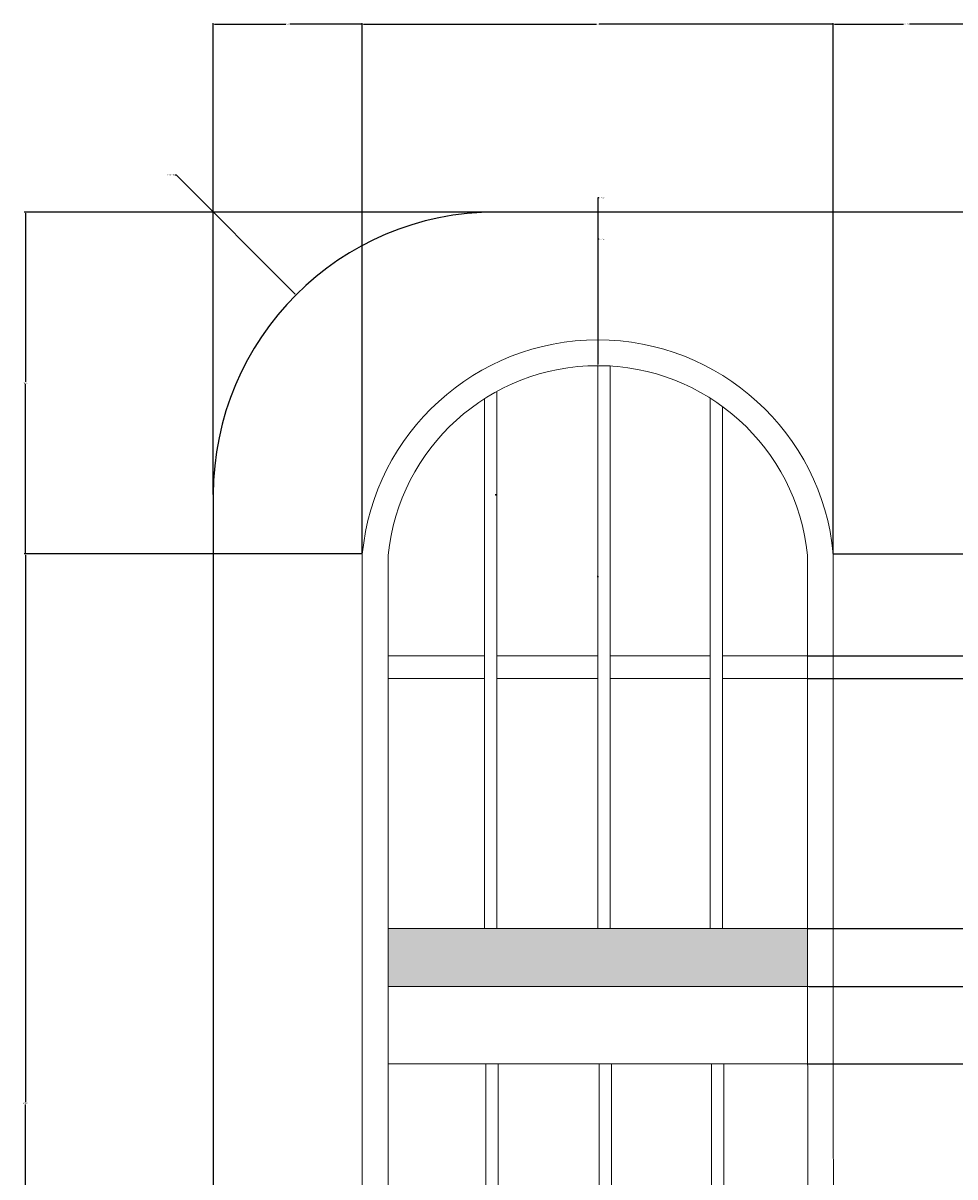
# Model space of a CAD drawing. Units: inches. Extents: x -14 to 375, y -86 to 549.
# Tile 10 of 12: x -14 to 130, y 336 to 515. Entities that reach past the tile are written whole.
import ezdxf

# ---------------------------------------------------------------- set-up
doc = ezdxf.new("R2010")
doc.units = ezdxf.units.IN
doc.header["$MEASUREMENT"] = 0
for name, color, linetype, lineweight in [('A-ANNO-DIMS', 2, 'Continuous', 18), ('A-ELEV', 7, 'Continuous', 25), ('A-ELEV-PATT', 8, 'Continuous', 13), ('A-GLAZ', 4, 'Continuous', 18)]:
    doc.layers.add(name, color=color, linetype=linetype, lineweight=lineweight)
doc.styles.get("Standard").update_dxf_attribs({"font": 'arial.ttf'})
doc.dimstyles.get("Standard").update_dxf_attribs({"dimtxt": 0.18, "dimasz": 0.18, "dimexe": 0.18, "dimexo": 0.0625, "dimgap": 0.09, "dimtad": 0, "dimtih": 1, "dimtoh": 1, "dimdec": 4, "dimzin": 0, "dimdsep": 46, "dimtxsty": 'Standard', "dimcen": 0.09, "dimadec": 0, "dimazin": 0, "dimtfac": 1, "dimtdec": 4, "dimtofl": 0, "dimtmove": 0, "dimatfit": 3, "dimfxl": 1, "dimtolj": 1, "dimtzin": 0, "dimarcsym": 0})

# ---------------------------------------------------------------- blocks, each defined once
blk = doc.blocks.new('*D5')
at = {"layer": 'A-ANNO-DIMS', "color": 0, "lineweight": -2, "transparency": 16777216}
for p, q in [((15.4, 442.21), (15.4, 515.24)), ((15.58, 515.06), (26.64, 515.06)), ((38.32, 515.06), (27.26, 515.06)), ((38.5, 433.03), (38.5, 515.24))]:
    blk.add_line(p, q, dxfattribs=at)
at = {"layer": 'A-ANNO-DIMS', "color": 0, "transparency": 16777216}
for points in [[(15.58, 515.09), (15.58, 515.03), (15.4, 515.06)], [(38.32, 515.09), (38.32, 515.03), (38.5, 515.06)]]:
    blk.add_solid(points, dxfattribs=at)
at = {"layer": 'Defpoints', "color": 0, "transparency": 16777216}
for p in [(38.5, 515.06), (15.4, 442.15), (38.5, 432.97)]:
    blk.add_point(p, dxfattribs=at)
at = {"layer": 'A-ANNO-DIMS', "color": 0, "transparency": 16777216, "insert": (26.95, 515.06), "char_height": 0.18, "attachment_point": 5}
blk.add_mtext('\\A1;23.1', dxfattribs=at)
blk = doc.blocks.new('*D6')
at = {"layer": 'A-ANNO-DIMS', "color": 0, "lineweight": -2, "transparency": 16777216}
for p, q in [((38.5, 433.03), (38.5, 515.24)), ((38.68, 515.06), (74.78, 515.06)), ((111.32, 515.06), (75.22, 515.06)), ((111.5, 433.03), (111.5, 515.24))]:
    blk.add_line(p, q, dxfattribs=at)
at = {"layer": 'A-ANNO-DIMS', "color": 0, "transparency": 16777216}
for points in [[(38.68, 515.09), (38.68, 515.03), (38.5, 515.06)], [(111.32, 515.09), (111.32, 515.03), (111.5, 515.06)]]:
    blk.add_solid(points, dxfattribs=at)
at = {"layer": 'Defpoints', "color": 0, "transparency": 16777216}
for p in [(111.5, 515.06), (38.5, 432.97), (111.5, 432.97)]:
    blk.add_point(p, dxfattribs=at)
at = {"layer": 'A-ANNO-DIMS', "color": 0, "transparency": 16777216, "insert": (75, 515.06), "char_height": 0.18, "attachment_point": 5}
blk.add_mtext('\\A1;73', dxfattribs=at)
blk = doc.blocks.new('*D7')
at = {"layer": 'A-ANNO-DIMS', "color": 0, "lineweight": -2, "transparency": 16777216}
for p, q in [((111.5, 433.03), (111.5, 515.24)), ((111.68, 515.06), (122.4, 515.06)), ((134.05, 515.06), (123.33, 515.06)), ((134.23, 433.23), (134.23, 515.24))]:
    blk.add_line(p, q, dxfattribs=at)
at = {"layer": 'A-ANNO-DIMS', "color": 0, "transparency": 16777216}
for points in [[(111.68, 515.09), (111.68, 515.03), (111.5, 515.06)], [(134.05, 515.09), (134.05, 515.03), (134.23, 515.06)]]:
    blk.add_solid(points, dxfattribs=at)
at = {"layer": 'Defpoints', "color": 0, "transparency": 16777216}
for p in [(134.23, 515.06), (111.5, 432.97), (134.23, 433.17)]:
    blk.add_point(p, dxfattribs=at)
at = {"layer": 'A-ANNO-DIMS', "color": 0, "transparency": 16777216, "insert": (122.87, 515.06), "char_height": 0.18, "attachment_point": 5}
blk.add_mtext('\\A1;22.735', dxfattribs=at)
blk = doc.blocks.new('*D17')
at = {"layer": 'A-ANNO-DIMS', "color": 0, "lineweight": -2, "transparency": 16777216}
for p, q in [((38.44, 432.97), (-13.88, 432.97)), ((-13.7, 432.79), (-13.7, 348.02)), ((-13.7, 262.89), (-13.7, 347.66)), ((134.17, 262.71), (-13.88, 262.71))]:
    blk.add_line(p, q, dxfattribs=at)
at = {"layer": 'A-ANNO-DIMS', "color": 0, "transparency": 16777216}
for points in [[(-13.73, 432.79), (-13.67, 432.79), (-13.7, 432.97)], [(-13.73, 262.89), (-13.67, 262.89), (-13.7, 262.71)]]:
    blk.add_solid(points, dxfattribs=at)
at = {"layer": 'Defpoints', "color": 0, "transparency": 16777216}
for p in [(-13.7, 432.97), (38.5, 432.97), (134.23, 262.71)]:
    blk.add_point(p, dxfattribs=at)
at = {"layer": 'A-ANNO-DIMS', "color": 0, "transparency": 16777216, "insert": (-13.7, 347.84), "char_height": 0.18, "attachment_point": 5}
blk.add_mtext('\\A1;170.26', dxfattribs=at)
blk = doc.blocks.new('*D18')
at = {"layer": 'A-ANNO-DIMS', "color": 0, "lineweight": -2, "transparency": 16777216}
for p, q in [((59.15, 485.96), (-13.88, 485.96)), ((-13.7, 485.78), (-13.7, 459.65)), ((-13.7, 433.15), (-13.7, 459.28)), ((38.44, 432.97), (-13.88, 432.97))]:
    blk.add_line(p, q, dxfattribs=at)
at = {"layer": 'A-ANNO-DIMS', "color": 0, "transparency": 16777216}
for points in [[(-13.73, 485.78), (-13.67, 485.78), (-13.7, 485.96)], [(-13.73, 433.15), (-13.67, 433.15), (-13.7, 432.97)]]:
    blk.add_solid(points, dxfattribs=at)
at = {"layer": 'Defpoints', "color": 0, "transparency": 16777216}
for p in [(-13.7, 485.96), (59.21, 485.96), (38.5, 432.97)]:
    blk.add_point(p, dxfattribs=at)
at = {"layer": 'A-ANNO-DIMS', "color": 0, "transparency": 16777216, "insert": (-13.7, 459.46), "char_height": 0.18, "attachment_point": 5}
blk.add_mtext('\\A1;52.99', dxfattribs=at)
blk = doc.blocks.new('*D36')
at = {"layer": 'A-ANNO-DIMS', "color": 0, "lineweight": -2, "transparency": 16777216}
for p, q in [((107.56, 353.96), (374.54, 353.96)), ((374.36, 353.78), (374.36, 327.93)), ((374.36, 301.72), (374.36, 327.57)), ((107.64, 301.54), (374.54, 301.54))]:
    blk.add_line(p, q, dxfattribs=at)
at = {"layer": 'A-ANNO-DIMS', "color": 0, "transparency": 16777216}
for points in [[(374.33, 353.78), (374.39, 353.78), (374.36, 353.96)], [(374.33, 301.72), (374.39, 301.72), (374.36, 301.54)]]:
    blk.add_solid(points, dxfattribs=at)
at = {"layer": 'Defpoints', "color": 0, "transparency": 16777216}
for p in [(107.5, 353.96), (374.36, 353.96), (107.58, 301.54)]:
    blk.add_point(p, dxfattribs=at)
at = {"layer": 'A-ANNO-DIMS', "color": 0, "transparency": 16777216, "insert": (374.36, 327.75), "char_height": 0.18, "attachment_point": 5}
blk.add_mtext('\\A1;52.42', dxfattribs=at)
blk = doc.blocks.new('*D37')
at = {"layer": 'A-ANNO-DIMS', "color": 0, "lineweight": -2, "transparency": 16777216}
for p, q in [((107.76, 365.96), (374.54, 365.96)), ((374.36, 365.78), (374.36, 360.14)), ((374.36, 354.14), (374.36, 359.78)), ((107.56, 353.96), (374.54, 353.96))]:
    blk.add_line(p, q, dxfattribs=at)
at = {"layer": 'A-ANNO-DIMS', "color": 0, "transparency": 16777216}
for points in [[(374.33, 365.78), (374.39, 365.78), (374.36, 365.96)], [(374.33, 354.14), (374.39, 354.14), (374.36, 353.96)]]:
    blk.add_solid(points, dxfattribs=at)
at = {"layer": 'Defpoints', "color": 0, "transparency": 16777216}
for p in [(107.7, 365.96), (374.36, 365.96), (107.5, 353.96)]:
    blk.add_point(p, dxfattribs=at)
at = {"layer": 'A-ANNO-DIMS', "color": 0, "transparency": 16777216, "insert": (374.36, 359.96), "char_height": 0.18, "attachment_point": 5}
blk.add_mtext('\\A1;12', dxfattribs=at)
blk = doc.blocks.new('*D38')
at = {"layer": 'A-ANNO-DIMS', "color": 0, "lineweight": -2, "transparency": 16777216}
for p, q in [((107.56, 374.96), (374.54, 374.96)), ((374.36, 374.78), (374.36, 370.64)), ((374.36, 366.14), (374.36, 370.28)), ((107.76, 365.96), (374.54, 365.96))]:
    blk.add_line(p, q, dxfattribs=at)
at = {"layer": 'A-ANNO-DIMS', "color": 0, "transparency": 16777216}
for points in [[(374.33, 374.78), (374.39, 374.78), (374.36, 374.96)], [(374.33, 366.14), (374.39, 366.14), (374.36, 365.96)]]:
    blk.add_solid(points, dxfattribs=at)
at = {"layer": 'Defpoints', "color": 0, "transparency": 16777216}
for p in [(107.5, 374.96), (374.36, 374.96), (107.7, 365.96)]:
    blk.add_point(p, dxfattribs=at)
at = {"layer": 'A-ANNO-DIMS', "color": 0, "transparency": 16777216, "insert": (374.36, 370.46), "char_height": 0.18, "attachment_point": 5}
blk.add_mtext('\\A1;9', dxfattribs=at)
blk = doc.blocks.new('*D39')
at = {"layer": 'A-ANNO-DIMS', "color": 0, "lineweight": -2, "transparency": 16777216}
for p, q in [((107.56, 413.68), (374.54, 413.68)), ((374.36, 413.5), (374.36, 394.5)), ((374.36, 375.14), (374.36, 394.14)), ((107.56, 374.96), (374.54, 374.96))]:
    blk.add_line(p, q, dxfattribs=at)
at = {"layer": 'A-ANNO-DIMS', "color": 0, "transparency": 16777216}
for points in [[(374.33, 413.5), (374.39, 413.5), (374.36, 413.68)], [(374.33, 375.14), (374.39, 375.14), (374.36, 374.96)]]:
    blk.add_solid(points, dxfattribs=at)
at = {"layer": 'Defpoints', "color": 0, "transparency": 16777216}
for p in [(107.5, 413.68), (374.36, 413.68), (107.5, 374.96)]:
    blk.add_point(p, dxfattribs=at)
at = {"layer": 'A-ANNO-DIMS', "color": 0, "transparency": 16777216, "insert": (374.36, 394.32), "char_height": 0.18, "attachment_point": 5}
blk.add_mtext('\\A1;38.72', dxfattribs=at)
blk = doc.blocks.new('*D40')
at = {"layer": 'A-ANNO-DIMS', "color": 0, "lineweight": -2, "transparency": 16777216}
for p, q in [((107.56, 417.18), (374.54, 417.18)), ((374.36, 417), (374.36, 415.61)), ((374.36, 413.86), (374.36, 415.25)), ((107.56, 413.68), (374.54, 413.68))]:
    blk.add_line(p, q, dxfattribs=at)
at = {"layer": 'A-ANNO-DIMS', "color": 0, "transparency": 16777216}
for points in [[(374.33, 417), (374.39, 417), (374.36, 417.18)], [(374.33, 413.86), (374.39, 413.86), (374.36, 413.68)]]:
    blk.add_solid(points, dxfattribs=at)
at = {"layer": 'Defpoints', "color": 0, "transparency": 16777216}
for p in [(107.5, 417.18), (374.36, 417.18), (107.5, 413.68)]:
    blk.add_point(p, dxfattribs=at)
at = {"layer": 'A-ANNO-DIMS', "color": 0, "transparency": 16777216, "insert": (374.36, 415.43), "char_height": 0.18, "attachment_point": 5}
blk.add_mtext('\\A1;3.501', dxfattribs=at)
blk = doc.blocks.new('*D41')
at = {"layer": 'A-ANNO-DIMS', "color": 0, "lineweight": -2, "transparency": 16777216}
for p, q in [((111.56, 432.97), (374.54, 432.97)), ((374.36, 432.79), (374.36, 425.26)), ((374.36, 417.36), (374.36, 424.89)), ((107.56, 417.18), (374.54, 417.18))]:
    blk.add_line(p, q, dxfattribs=at)
at = {"layer": 'A-ANNO-DIMS', "color": 0, "transparency": 16777216}
for points in [[(374.33, 432.79), (374.39, 432.79), (374.36, 432.97)], [(374.33, 417.36), (374.39, 417.36), (374.36, 417.18)]]:
    blk.add_solid(points, dxfattribs=at)
at = {"layer": 'Defpoints', "color": 0, "transparency": 16777216}
for p in [(111.5, 432.97), (374.36, 432.97), (107.5, 417.18)]:
    blk.add_point(p, dxfattribs=at)
at = {"layer": 'A-ANNO-DIMS', "color": 0, "transparency": 16777216, "insert": (374.36, 425.07), "char_height": 0.18, "attachment_point": 5}
blk.add_mtext('\\A1;15.786', dxfattribs=at)
blk = doc.blocks.new('*D130')
at = {"layer": 'A-ANNO-DIMS', "color": 0, "lineweight": -2, "transparency": 16777216}
for p, q in [((9.47, 491.71), (9.65, 491.71)), ((9.65, 491.71), (28.11, 473.25)), ((59.12, 442.15), (59.3, 442.15)), ((59.21, 442.06), (59.21, 442.24))]:
    blk.add_line(p, q, dxfattribs=at)
at = {"layer": 'A-ANNO-DIMS', "color": 0, "transparency": 16777216}
blk.add_solid([(28.13, 473.28), (28.08, 473.23), (28.23, 473.13)], dxfattribs=at)
at = {"layer": 'Defpoints', "color": 0, "transparency": 16777216}
for p in [(28.23, 473.13), (59.21, 442.15)]:
    blk.add_point(p, dxfattribs=at)
at = {"layer": 'A-ANNO-DIMS', "color": 0, "transparency": 16777216, "insert": (8.81, 491.71), "char_height": 0.18, "attachment_point": 5}
blk.add_mtext('\\A1;2X R43.81', dxfattribs=at)
blk = doc.blocks.new('*D131')
at = {"layer": 'A-ANNO-DIMS', "color": 0, "lineweight": -2, "transparency": 16777216}
for p, q in [((75.18, 488.15), (75, 488.15)), ((75, 488.15), (75, 466.33)), ((74.91, 429.49), (75.09, 429.49)), ((75, 429.4), (75, 429.58))]:
    blk.add_line(p, q, dxfattribs=at)
at = {"layer": 'A-ANNO-DIMS', "color": 0, "transparency": 16777216}
blk.add_solid([(74.97, 466.33), (75.03, 466.33), (75, 466.15)], dxfattribs=at)
at = {"layer": 'Defpoints', "color": 0, "transparency": 16777216}
for p in [(75, 466.15), (75, 429.49)]:
    blk.add_point(p, dxfattribs=at)
at = {"layer": 'A-ANNO-DIMS', "color": 0, "transparency": 16777216, "insert": (75.66, 488.15), "char_height": 0.18, "attachment_point": 5}
blk.add_mtext('\\A1;R36.66', dxfattribs=at)
blk = doc.blocks.new('*D132')
at = {"layer": 'A-ANNO-DIMS', "color": 0, "lineweight": -2, "transparency": 16777216}
for p, q in [((75.18, 481.75), (75, 481.75)), ((75, 481.75), (75, 462.33)), ((74.91, 429.49), (75.09, 429.49)), ((75, 429.4), (75, 429.58))]:
    blk.add_line(p, q, dxfattribs=at)
at = {"layer": 'A-ANNO-DIMS', "color": 0, "transparency": 16777216}
blk.add_solid([(74.97, 462.33), (75.03, 462.33), (75, 462.15)], dxfattribs=at)
at = {"layer": 'Defpoints', "color": 0, "transparency": 16777216}
for p in [(75, 462.15), (75, 429.49)]:
    blk.add_point(p, dxfattribs=at)
at = {"layer": 'A-ANNO-DIMS', "color": 0, "transparency": 16777216, "insert": (75.66, 481.75), "char_height": 0.18, "attachment_point": 5}
blk.add_mtext('\\A1;R32.66', dxfattribs=at)

msp = doc.modelspace()

# ---------------------------------------------------------------- hatches: boundary and pattern name
at = {"layer": 'A-ELEV-PATT'}
h = msp.add_hatch(dxfattribs=at)
h.set_pattern_fill('SWAMP', color=256, scale=0.8)
h.set_pattern_definition([(0, (-168.40604, -22.7026), (0.4, 0.6928203), [0.1, -0.7]), (90, (-168.35604, -22.7026), (-0.4, 0.69282032), [0.05, -1.3356406]), (90, (-168.34354, -22.7026), (-0.4, 0.69282032), [0.04, -1.3456406]), (90, (-168.36854, -22.7026), (-0.4, 0.69282032), [0.04, -1.3456406]), (60, (-168.33104, -22.7026), (-0.4, 0.6928203), [0.032, -0.768]), (120, (-168.38104, -22.7026), (-0.8, 3e-10), [0.032, -0.768])])
h.paths.add_polyline_path([(42.5033, 374.9589), (42.5033, 365.9589), (107.4987, 365.9589), (107.4987, 374.9589)])
h.paths.add_polyline_path([(107.615, 245.9589), (107.6063, 254.9589), (42.5033, 254.9589), (42.5033, 245.9589)])

# ---------------------------------------------------------------- linework, layer by layer
at = {"layer": 'A-ELEV'}
for p, q in [((301.4553, 485.9589), (59.2112, 485.9589)), ((15.4018, 442.1495), (15.4018, 365.9589)), ((15.4018, 365.9589), (15.4018, 245.9589))]:
    msp.add_line(p, q, dxfattribs=at)
msp.add_arc((59.2112, 442.1495), 43.8094, 90, 180, dxfattribs=at)
at = {"layer": 'A-GLAZ'}
for p, q in [((42.5033, 374.9589), (107.4987, 374.9589)), ((107.4899, 374.9589), (107.7019, 156.3768)), ((42.5033, 365.9589), (107.7019, 365.9589)), ((107.7019, 365.9589), (42.5033, 365.9589)), ((42.5033, 365.9589), (107.4987, 365.9589)), ((42.5033, 353.9589), (107.4987, 353.9589)), ((57.6445, 254.9589), (57.6445, 353.9589)), ((59.5668, 353.9589), (59.5668, 254.9589)), ((75.2042, 254.9589), (75.2042, 353.9589)), ((77.1265, 353.9589), (77.1265, 254.9589)), ((92.5999, 254.9589), (92.5999, 353.9589)), ((94.5222, 353.9589), (94.5222, 254.9589))]:
    msp.add_line(p, q, dxfattribs=at)
for points in [[(111.4987, 365.9589), (111.7019, 152.3768), (38.5033, 152.3768), (38.5033, 365.9589), (38.5033, 432.9679, -0.90920588), (111.4987, 432.9679), (111.4987, 365.9589)], [(42.5033, 156.3768), (42.5033, 365.9589), (42.5033, 432.7722, -0.9040533), (107.4987, 432.7722), (107.4987, 365.9589)]]:
    msp.add_lwpolyline(points, format="xyb", dxfattribs=at)
msp.add_lwpolyline([(75.001, 462.1518), (76.9233, 462.1518), (76.9233, 374.9589), (75.001, 374.9589)], close=True, dxfattribs=at)
for points in [[(59.3636, 458.1653), (59.3636, 374.9589), (57.4413, 374.9589), (57.4413, 457.0302)], [(94.319, 455.8268), (94.319, 374.9589), (92.3967, 374.9589), (92.3967, 457.1341)], [(57.4413, 417.1817), (42.5033, 417.1817), (42.5033, 413.6806), (57.4413, 413.6806)], [(75.001, 417.1817), (59.3636, 417.1817)], [(92.3967, 417.1817), (76.9233, 417.1817)], [(94.319, 413.6806), (107.4987, 413.6806), (107.4987, 417.1817), (94.319, 417.1817)], [(59.3636, 413.6806), (75.001, 413.6806)], [(76.9233, 413.6806), (92.3967, 413.6806)]]:
    msp.add_lwpolyline(points, dxfattribs=at)

# ---------------------------------------------------------------- dimensions: what is measured, and where the dimension line sits
at = {"layer": 'A-ANNO-DIMS'}
for base, p1, p2, override, picture, middle in [((38.5033, 515.0589), (15.4018, 442.1495), (38.5033, 432.9679), {"dimdec": 1, "dimlfac": 1, "dimrnd": 0, "dimzin": 0, "dimdsep": 46, "dimlunit": 2}, '*D5', (26.9526, 515.0589)), ((111.4987, 515.0589), (38.5033, 432.9679), (111.4987, 432.9679), {"dimdec": 0, "dimlfac": 1, "dimrnd": 0, "dimzin": 0, "dimdsep": 46, "dimlunit": 2}, '*D6', (75.001, 515.0589)), ((134.2334, 515.0589), (111.4987, 432.9679), (134.2334, 433.1717), {"dimdec": 3, "dimlfac": 1, "dimrnd": 0, "dimzin": 0, "dimdsep": 46, "dimlunit": 2}, '*D7', (122.866, 515.0589))]:
    dim = msp.add_linear_dim(base=base, p1=p1, p2=p2, dimstyle='Standard', override=override, dxfattribs=at)
    dim.commit()
    dim.dimension.update_dxf_attribs({"geometry": picture, "text_midpoint": middle})
dim = msp.add_radius_dim(center=(59.2112, 442.1495), mpoint=(28.2329, 473.1271), text='2X <>', dimstyle='Standard', override={"dimdec": 2, "dimlfac": 1, "dimrnd": 0, "dimzin": 0, "dimdsep": 46, "dimlunit": 2}, dxfattribs=at)
dim.commit()
dim.dimension.update_dxf_attribs({"geometry": '*D130', "text_midpoint": (8.8086, 491.7136), "dimtype": 164})
for mpoint, picture, middle in [((75.001, 466.1518), '*D131', (75.6608, 488.1497)), ((75.001, 462.1518), '*D132', (75.6608, 481.7497))]:
    dim = msp.add_radius_dim(center=(75.001, 429.4887), mpoint=mpoint, dimstyle='Standard', override={"dimdec": 2, "dimlfac": 1, "dimrnd": 0, "dimzin": 0, "dimdsep": 46, "dimlunit": 2}, dxfattribs=at)
    dim.commit()
    dim.dimension.update_dxf_attribs({"geometry": picture, "text_midpoint": middle, "dimtype": 164})
for base, p1, p2, override, picture, middle in [((-13.6982, 485.9589), (38.5033, 432.9679), (59.2112, 485.9589), {"dimdec": 2, "dimlfac": 1, "dimrnd": 0, "dimzin": 0, "dimdsep": 46, "dimlunit": 2}, '*D18', (-13.6982, 459.4634)), ((-13.6982, 432.9679), (134.2334, 262.7071), (38.5033, 432.9679), {"dimdec": 2, "dimlfac": 1, "dimrnd": 0, "dimzin": 0, "dimdsep": 46, "dimlunit": 2}, '*D17', (-13.6982, 347.8375)), ((374.3647, 432.9679), (107.4987, 417.1817), (111.4987, 432.9679), {"dimdec": 3, "dimlfac": 1, "dimrnd": 0, "dimzin": 0, "dimdsep": 46, "dimlunit": 2}, '*D41', (374.3647, 425.0748)), ((374.3647, 417.1817), (107.4987, 413.6806), (107.4987, 417.1817), {"dimdec": 3, "dimlfac": 1, "dimrnd": 0, "dimzin": 0, "dimdsep": 46, "dimlunit": 2}, '*D40', (374.3647, 415.4312)), ((374.3647, 413.6806), (107.4987, 374.9589), (107.4987, 413.6806), {"dimdec": 2, "dimlfac": 1, "dimrnd": 0, "dimzin": 0, "dimdsep": 46, "dimlunit": 2}, '*D39', (374.3647, 394.3198)), ((374.3647, 374.9589), (107.7019, 365.9589), (107.4987, 374.9589), {"dimdec": 0, "dimlfac": 1, "dimrnd": 0, "dimzin": 0, "dimdsep": 46, "dimlunit": 2}, '*D38', (374.3647, 370.4589)), ((374.3647, 365.9589), (107.4987, 353.9589), (107.7019, 365.9589), {"dimdec": 0, "dimlfac": 1, "dimrnd": 0, "dimzin": 0, "dimdsep": 46, "dimlunit": 2}, '*D37', (374.3647, 359.9589)), ((374.3647, 353.9589), (107.5784, 301.5363), (107.4987, 353.9589), {"dimdec": 2, "dimlfac": 1, "dimrnd": 0, "dimzin": 0, "dimdsep": 46, "dimlunit": 2}, '*D36', (374.3647, 327.7476))]:
    dim = msp.add_linear_dim(base=base, p1=p1, p2=p2, angle=90, dimstyle='Standard', override=override, dxfattribs=at)
    dim.commit()
    dim.dimension.update_dxf_attribs({"geometry": picture, "text_midpoint": middle})

doc.saveas('drawing.dxf')
